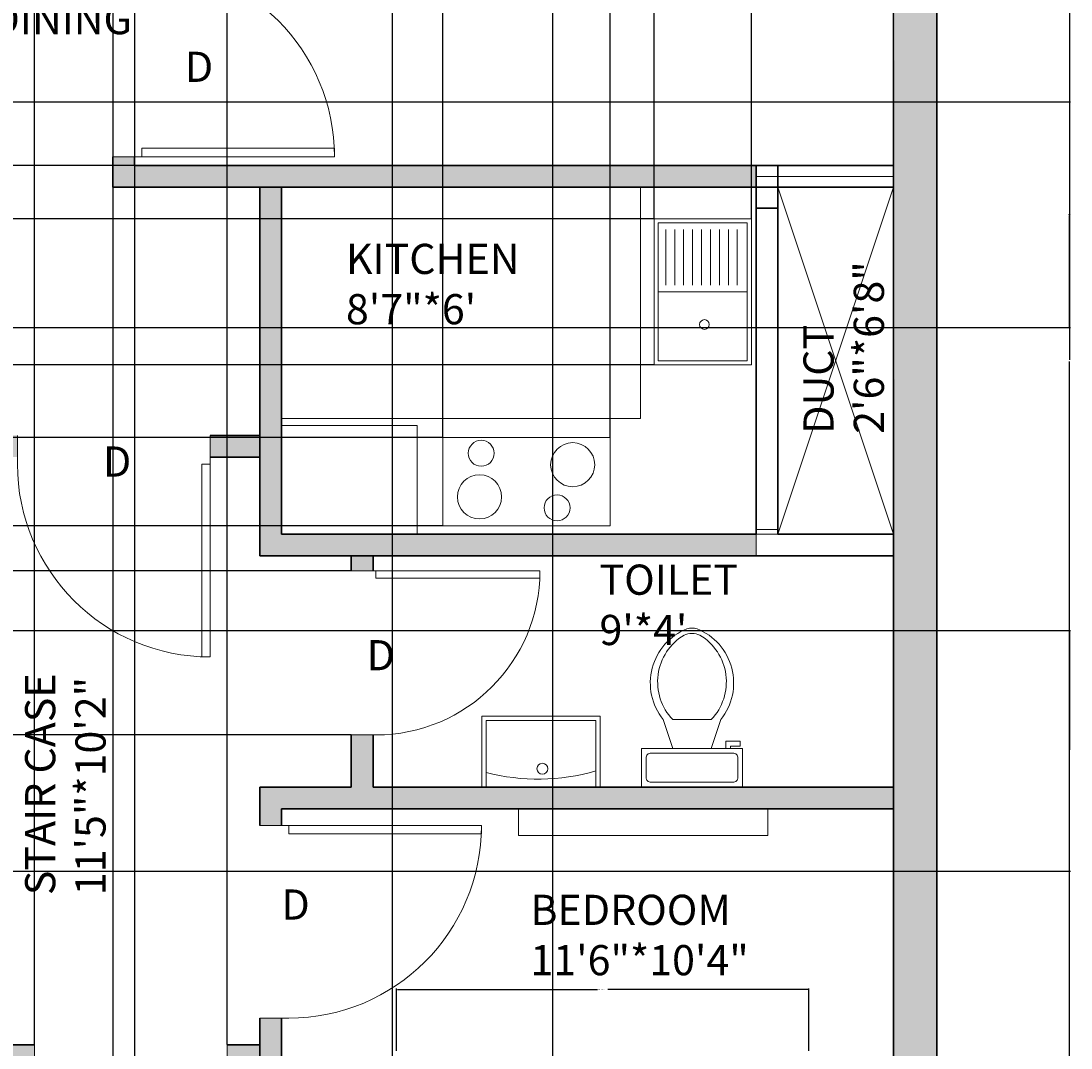
# Model space of a CAD drawing. Units: inches. Extents: x 1841 to 2210, y 2173 to 2736.
# Tile 3 of 4: x 1979 to 2197, y 2316 to 2529. Entities that reach past the tile are written whole.
import ezdxf

# ---------------------------------------------------------------- set-up
doc = ezdxf.new("R2010")
doc.units = ezdxf.units.IN
for name, color, linetype, lineweight in [('A-ANNO-DIMS', 2, 'Continuous', 18), ('A-AREA-IDEN', 10, 'Continuous', 18), ('A-EQPM', 8, 'Continuous', 18), ('A-FLOR-CABN', 8, 'Continuous', 18), ('A-FLOR-FIXT', 9, 'Continuous', 18), ('A-FLOR-FIXT-PATT', 9, 'Continuous', 13), ('A-FLOR-OPEN', 8, 'Continuous', 18), ('A-FURN', 8, 'Continuous', 18), ('A-WALL', 7, 'Continuous', 35), ('A-WALL-PATT', 252, 'Continuous', 13), ('DOOR', 50, 'Continuous', 18), ('TEXT', 10, 'Continuous', 18), ('WIN', 193, 'Continuous', 18)]:
    doc.layers.add(name, color=color, linetype=linetype, lineweight=lineweight)
doc.styles.get("Standard").update_dxf_attribs({"font": 'arial.ttf'})
doc.dimstyles.get("Standard").update_dxf_attribs({"dimtxt": 0.18, "dimasz": 0.18, "dimexe": 0.18, "dimexo": 0.0625, "dimgap": 0.09, "dimtad": 0, "dimtih": 1, "dimtoh": 1, "dimdec": 4, "dimzin": 0, "dimdsep": 46, "dimtxsty": 'Standard', "dimcen": 0.09, "dimadec": 0, "dimazin": 0, "dimtfac": 1, "dimtdec": 4, "dimtofl": 0, "dimtmove": 0, "dimatfit": 3, "dimfxl": 1, "dimtolj": 1, "dimtzin": 0, "dimarcsym": 0})

# ---------------------------------------------------------------- blocks, each defined once
blk = doc.blocks.new('*U2')
for p, q in [((0, 0), (0, -6)), ((40, 0), (40, -6))]:
    blk.add_line(p, q)
blk.add_lwpolyline([(0, 0), (0, 40), (1.75, 40), (1.75, 0)], close=True)
blk.add_arc((0, 0), 40, 0, 90)
blk = doc.blocks.new('*U4')
for p, q in [((9.5, -6), (9.5, -2)), ((-10, -8.5), (-8, -8.5)), ((-10, -9.5), (-10, -8.5)), ((-8, -8.5), (-8, -8)), ((-7, -8), (-7, -9.5)), ((-4, -8), (-6, -14)), ((4, -8), (6, -14)), ((-7, -9.5), (-10, -9.5)), ((4, -14), (-4, -14))]:
    blk.add_line(p, q)
blk.add_lwpolyline([(10.5, -8), (10.5, 0), (-10.5, 0), (-10.5, -8)], close=True)
for points in [[(-9.5, -2), (-9.5, -6)], [(8.5, -1), (-8.5, -1)], [(-8.5, -7), (8.5, -7)]]:
    blk.add_lwpolyline(points)
for centre, radius, start, end in [((-8.62, -1.88), 0.884, 81.8699, 188.1301), ((8.62, -1.88), 0.884, 351.8699, 98.1301), ((-8.62, -6.12), 0.884, 171.8699, 278.1301), ((8.62, -6.12), 0.884, 261.8699, 8.1301), ((3.52, -21.58), 12.17, 141.4691, 247.9714), ((4.2, -21.82), 11.33, 136.3677, 238.9468), ((-3.52, -21.58), 12.17, 292.0284, 38.5307), ((-4.2, -21.82), 11.33, 301.053, 43.6321), ((0, -27.88), 4, 245.7318, 294.2682), ((0, -29), 4, 254.8605, 285.1395)]:
    blk.add_arc(centre, radius, start, end)
blk = doc.blocks.new('BASIN-WALL')
blk.add_lwpolyline([(24.58, 14.71), (24.58, 0), (0, 0), (0, 14.71)])
blk.add_lwpolyline([(0.91, 14.71), (23.68, 14.71), (23.68, 0.91), (0.91, 0.91)], close=True)
blk.add_circle((11.97, 10.91), 1.13)
blk.add_arc((12.85, -29.32), 42.4, 75.2054, 106.3847)
blk = doc.blocks.new('*D16')
at = {"layer": 'A-ANNO-DIMS', "color": 0, "lineweight": -2, "transparency": 16777216}
for p, q in [((2056.93, 2315.11), (2056.93, 2328.07)), ((2057.11, 2327.89), (2098.62, 2327.89)), ((2142.32, 2327.89), (2100.81, 2327.89)), ((2142.5, 2315.11), (2142.5, 2328.07))]:
    blk.add_line(p, q, dxfattribs=at)
at = {"layer": 'A-ANNO-DIMS', "color": 0, "transparency": 16777216}
for points in [[(2057.11, 2327.92), (2057.11, 2327.86), (2056.93, 2327.89)], [(2142.32, 2327.92), (2142.32, 2327.86), (2142.5, 2327.89)]]:
    blk.add_solid(points, dxfattribs=at)
at = {"layer": 'Defpoints', "color": 0, "transparency": 16777216}
for p in [(2056.93, 2327.89), (2056.93, 2315.05), (2142.5, 2315.05)]:
    blk.add_point(p, dxfattribs=at)
at = {"layer": 'A-ANNO-DIMS', "color": 0, "transparency": 16777216, "insert": (2099.72, 2327.89), "char_height": 0.18, "attachment_point": 5}
blk.add_mtext('\\A1;BED SET 86 TYP.', dxfattribs=at)
blk = doc.blocks.new('*D23')
at = {"layer": 'A-ANNO-DIMS', "color": 0, "lineweight": -2, "transparency": 16777216}
for p, q in [((2169.11, 2708.41), (2196.78, 2708.41)), ((2196.6, 2708.23), (2196.6, 2458.59)), ((2196.6, 2208.59), (2196.6, 2458.22)), ((2028.61, 2208.41), (2196.78, 2208.41))]:
    blk.add_line(p, q, dxfattribs=at)
at = {"layer": 'A-ANNO-DIMS', "color": 0, "transparency": 16777216}
for points in [[(2196.57, 2708.23), (2196.63, 2708.23), (2196.6, 2708.41)], [(2196.57, 2208.59), (2196.63, 2208.59), (2196.6, 2208.41)]]:
    blk.add_solid(points, dxfattribs=at)
at = {"layer": 'Defpoints', "color": 0, "transparency": 16777216}
for p in [(2169.05, 2708.41), (2196.6, 2708.41), (2028.55, 2208.41)]:
    blk.add_point(p, dxfattribs=at)
at = {"layer": 'A-ANNO-DIMS', "color": 0, "transparency": 16777216, "insert": (2196.6, 2458.41), "char_height": 0.18, "attachment_point": 5}
blk.add_mtext('\\A1;500', dxfattribs=at)
blk = doc.blocks.new('*D35')
at = {"layer": 'A-ANNO-DIMS', "color": 0, "lineweight": -2, "transparency": 16777216}
for p, q in [((2159.99, 2546.82), (1841.32, 2546.82)), ((1841.5, 2546.64), (1841.5, 2523.04)), ((1841.5, 2499.09), (1841.5, 2522.68)), ((2159.99, 2498.91), (1841.32, 2498.91))]:
    blk.add_line(p, q, dxfattribs=at)
at = {"layer": 'A-ANNO-DIMS', "color": 0, "transparency": 16777216}
for points in [[(1841.47, 2546.64), (1841.53, 2546.64), (1841.5, 2546.82)], [(1841.47, 2499.09), (1841.53, 2499.09), (1841.5, 2498.91)]]:
    blk.add_solid(points, dxfattribs=at)
at = {"layer": 'Defpoints', "color": 0, "transparency": 16777216}
for p in [(1841.5, 2546.82), (2160.05, 2546.82), (2160.05, 2498.91)]:
    blk.add_point(p, dxfattribs=at)
at = {"layer": 'A-ANNO-DIMS', "color": 0, "transparency": 16777216, "insert": (1841.5, 2522.86), "char_height": 0.18, "attachment_point": 5}
blk.add_mtext('\\A1;47.91', dxfattribs=at)
blk = doc.blocks.new('*D36')
at = {"layer": 'A-ANNO-DIMS', "color": 0, "lineweight": -2, "transparency": 16777216}
for p, q in [((1981.8, 2316.47), (1981.8, 2736.14)), ((1981.98, 2735.96), (2001.58, 2735.96)), ((2021.62, 2735.96), (2002.02, 2735.96)), ((2021.8, 2316.47), (2021.8, 2736.14))]:
    blk.add_line(p, q, dxfattribs=at)
at = {"layer": 'A-ANNO-DIMS', "color": 0, "transparency": 16777216}
for points in [[(1981.98, 2735.99), (1981.98, 2735.93), (1981.8, 2735.96)], [(2021.62, 2735.99), (2021.62, 2735.93), (2021.8, 2735.96)]]:
    blk.add_solid(points, dxfattribs=at)
at = {"layer": 'Defpoints', "color": 0, "transparency": 16777216}
for p in [(2021.8, 2735.96), (1981.8, 2316.41), (2021.8, 2316.41)]:
    blk.add_point(p, dxfattribs=at)
at = {"layer": 'A-ANNO-DIMS', "color": 0, "transparency": 16777216, "insert": (2001.8, 2735.96), "char_height": 0.18, "attachment_point": 5}
blk.add_mtext('\\A1;40', dxfattribs=at)
blk = doc.blocks.new('*D39')
at = {"layer": 'A-ANNO-DIMS', "color": 0, "lineweight": -2, "transparency": 16777216}
for p, q in [((1914.11, 2402.41), (2196.78, 2402.41)), ((2196.6, 2402.23), (2196.6, 2377.59)), ((2196.6, 2352.59), (2196.6, 2377.22)), ((1914.11, 2352.41), (2196.78, 2352.41))]:
    blk.add_line(p, q, dxfattribs=at)
at = {"layer": 'A-ANNO-DIMS', "color": 0, "transparency": 16777216}
for points in [[(2196.57, 2402.23), (2196.63, 2402.23), (2196.6, 2402.41)], [(2196.57, 2352.59), (2196.63, 2352.59), (2196.6, 2352.41)]]:
    blk.add_solid(points, dxfattribs=at)
at = {"layer": 'Defpoints', "color": 0, "transparency": 16777216}
for p in [(1914.05, 2402.41), (2196.6, 2402.41), (1914.05, 2352.41)]:
    blk.add_point(p, dxfattribs=at)
at = {"layer": 'A-ANNO-DIMS', "color": 0, "transparency": 16777216, "insert": (2196.6, 2377.41), "char_height": 0.18, "attachment_point": 5}
blk.add_mtext('\\A1;50', dxfattribs=at)
blk = doc.blocks.new('*D41')
at = {"layer": 'A-ANNO-DIMS', "color": 0, "lineweight": -2, "transparency": 16777216}
for p, q in [((1938.73, 2512.15), (2196.78, 2512.15)), ((2196.6, 2511.97), (2196.6, 2488.89)), ((2196.6, 2465.46), (2196.6, 2488.53)), ((1938.73, 2465.28), (2196.78, 2465.28))]:
    blk.add_line(p, q, dxfattribs=at)
at = {"layer": 'A-ANNO-DIMS', "color": 0, "transparency": 16777216}
for points in [[(2196.57, 2511.97), (2196.63, 2511.97), (2196.6, 2512.15)], [(2196.57, 2465.46), (2196.63, 2465.46), (2196.6, 2465.28)]]:
    blk.add_solid(points, dxfattribs=at)
at = {"layer": 'Defpoints', "color": 0, "transparency": 16777216}
for p in [(1938.67, 2512.15), (2196.6, 2512.15), (1938.67, 2465.28)]:
    blk.add_point(p, dxfattribs=at)
at = {"layer": 'A-ANNO-DIMS', "color": 0, "transparency": 16777216, "insert": (2196.6, 2488.71), "char_height": 0.18, "attachment_point": 5}
blk.add_mtext('\\A1;46.87', dxfattribs=at)
blk = doc.blocks.new('*D43')
at = {"layer": 'A-ANNO-DIMS', "color": 0, "lineweight": -2, "transparency": 16777216}
for p, q in [((2056.06, 2637.84), (2056.06, 2180.68)), ((2089.3, 2637.84), (2089.3, 2180.68)), ((2056.24, 2180.86), (2072.22, 2180.86)), ((2089.12, 2180.86), (2073.14, 2180.86))]:
    blk.add_line(p, q, dxfattribs=at)
at = {"layer": 'A-ANNO-DIMS', "color": 0, "transparency": 16777216}
for points in [[(2056.24, 2180.89), (2056.24, 2180.83), (2056.06, 2180.86)], [(2089.12, 2180.89), (2089.12, 2180.83), (2089.3, 2180.86)]]:
    blk.add_solid(points, dxfattribs=at)
at = {"layer": 'Defpoints', "color": 0, "transparency": 16777216}
for p in [(2056.06, 2637.91), (2089.3, 2637.91), (2089.3, 2180.86)]:
    blk.add_point(p, dxfattribs=at)
at = {"layer": 'A-ANNO-DIMS', "color": 0, "transparency": 16777216, "insert": (2072.68, 2180.86), "char_height": 0.18, "attachment_point": 5}
blk.add_mtext('\\A1;33.234', dxfattribs=at)
blk = doc.blocks.new('*D44')
at = {"layer": 'A-ANNO-DIMS', "color": 0, "lineweight": -2, "transparency": 16777216}
for p, q in [((2047.49, 2414.75), (1841.32, 2414.75)), ((1841.5, 2414.57), (1841.5, 2397.92)), ((1841.5, 2380.9), (1841.5, 2397.56)), ((2047.49, 2380.72), (1841.32, 2380.72))]:
    blk.add_line(p, q, dxfattribs=at)
at = {"layer": 'A-ANNO-DIMS', "color": 0, "transparency": 16777216}
for points in [[(1841.47, 2414.57), (1841.53, 2414.57), (1841.5, 2414.75)], [(1841.47, 2380.9), (1841.53, 2380.9), (1841.5, 2380.72)]]:
    blk.add_solid(points, dxfattribs=at)
at = {"layer": 'Defpoints', "color": 0, "transparency": 16777216}
for p in [(1841.5, 2414.75), (2047.55, 2414.75), (2047.55, 2380.72)]:
    blk.add_point(p, dxfattribs=at)
at = {"layer": 'A-ANNO-DIMS', "color": 0, "transparency": 16777216, "insert": (1841.5, 2397.74), "char_height": 0.18, "attachment_point": 5}
blk.add_mtext('\\A1;34.03', dxfattribs=at)
blk = doc.blocks.new('*D45')
at = {"layer": 'A-ANNO-DIMS', "color": 0, "lineweight": -2, "transparency": 16777216}
for p, q in [((1998.05, 2540.69), (1998.05, 2180.68)), ((2002.55, 2540.69), (2002.55, 2180.68)), ((1998.23, 2180.86), (2000.04, 2180.86)), ((2002.37, 2180.86), (2000.56, 2180.86))]:
    blk.add_line(p, q, dxfattribs=at)
at = {"layer": 'A-ANNO-DIMS', "color": 0, "transparency": 16777216}
for points in [[(1998.23, 2180.89), (1998.23, 2180.83), (1998.05, 2180.86)], [(2002.37, 2180.89), (2002.37, 2180.83), (2002.55, 2180.86)]]:
    blk.add_solid(points, dxfattribs=at)
at = {"layer": 'Defpoints', "color": 0, "transparency": 16777216}
for p in [(1998.05, 2540.75), (2002.55, 2540.75), (2002.55, 2180.86)]:
    blk.add_point(p, dxfattribs=at)
at = {"layer": 'A-ANNO-DIMS', "color": 0, "transparency": 16777216, "insert": (2000.3, 2180.86), "char_height": 0.18, "attachment_point": 5}
blk.add_mtext('\\A1;4.5', dxfattribs=at)
blk = doc.blocks.new('*D47')
at = {"layer": 'A-ANNO-DIMS', "color": 0, "lineweight": -2, "transparency": 16777216}
for p, q in [((2066.54, 2442.55), (2066.54, 2736.14)), ((2066.72, 2735.96), (2083.52, 2735.96)), ((2101.11, 2735.96), (2084.31, 2735.96)), ((2101.29, 2442.55), (2101.29, 2736.14))]:
    blk.add_line(p, q, dxfattribs=at)
at = {"layer": 'A-ANNO-DIMS', "color": 0, "transparency": 16777216}
for points in [[(2066.72, 2735.99), (2066.72, 2735.93), (2066.54, 2735.96)], [(2101.11, 2735.99), (2101.11, 2735.93), (2101.29, 2735.96)]]:
    blk.add_solid(points, dxfattribs=at)
at = {"layer": 'Defpoints', "color": 0, "transparency": 16777216}
for p in [(2101.29, 2735.96), (2066.54, 2442.49), (2101.29, 2442.49)]:
    blk.add_point(p, dxfattribs=at)
at = {"layer": 'A-ANNO-DIMS', "color": 0, "transparency": 16777216, "insert": (2083.91, 2735.96), "char_height": 0.18, "attachment_point": 5}
blk.add_mtext('\\A1;34.75', dxfattribs=at)
blk = doc.blocks.new('*D48')
at = {"layer": 'A-ANNO-DIMS', "color": 0, "lineweight": -2, "transparency": 16777216}
for p, q in [((2066.48, 2442.49), (1841.32, 2442.49)), ((1841.5, 2442.31), (1841.5, 2433.48)), ((1841.5, 2424.29), (1841.5, 2433.12)), ((2066.48, 2424.11), (1841.32, 2424.11))]:
    blk.add_line(p, q, dxfattribs=at)
at = {"layer": 'A-ANNO-DIMS', "color": 0, "transparency": 16777216}
for points in [[(1841.47, 2442.31), (1841.53, 2442.31), (1841.5, 2442.49)], [(1841.47, 2424.29), (1841.53, 2424.29), (1841.5, 2424.11)]]:
    blk.add_solid(points, dxfattribs=at)
at = {"layer": 'Defpoints', "color": 0, "transparency": 16777216}
for p in [(1841.5, 2442.49), (2066.54, 2442.49), (2066.54, 2424.11)]:
    blk.add_point(p, dxfattribs=at)
at = {"layer": 'A-ANNO-DIMS', "color": 0, "transparency": 16777216, "insert": (1841.5, 2433.3), "char_height": 0.18, "attachment_point": 5}
blk.add_mtext('\\A1;18.377', dxfattribs=at)
blk = doc.blocks.new('*D49')
at = {"layer": 'A-ANNO-DIMS', "color": 0, "lineweight": -2, "transparency": 16777216}
for p, q in [((2110.38, 2487.94), (2110.38, 2736.14)), ((2110.56, 2735.96), (2120.1, 2735.96)), ((2130.41, 2735.96), (2120.86, 2735.96)), ((2130.59, 2487.94), (2130.59, 2736.14))]:
    blk.add_line(p, q, dxfattribs=at)
at = {"layer": 'A-ANNO-DIMS', "color": 0, "transparency": 16777216}
for points in [[(2110.56, 2735.99), (2110.56, 2735.93), (2110.38, 2735.96)], [(2130.41, 2735.99), (2130.41, 2735.93), (2130.59, 2735.96)]]:
    blk.add_solid(points, dxfattribs=at)
at = {"layer": 'Defpoints', "color": 0, "transparency": 16777216}
for p in [(2130.59, 2735.96), (2110.38, 2487.88), (2130.59, 2487.88)]:
    blk.add_point(p, dxfattribs=at)
at = {"layer": 'A-ANNO-DIMS', "color": 0, "transparency": 16777216, "insert": (2120.48, 2735.96), "char_height": 0.18, "attachment_point": 5}
blk.add_mtext('\\A1;20.21', dxfattribs=at)
blk = doc.blocks.new('*D50')
at = {"layer": 'A-ANNO-DIMS', "color": 0, "lineweight": -2, "transparency": 16777216}
for p, q in [((2110.31, 2487.88), (1841.32, 2487.88)), ((1841.5, 2487.7), (1841.5, 2472.88)), ((1841.5, 2457.7), (1841.5, 2472.52)), ((2110.31, 2457.52), (1841.32, 2457.52))]:
    blk.add_line(p, q, dxfattribs=at)
at = {"layer": 'A-ANNO-DIMS', "color": 0, "transparency": 16777216}
for points in [[(1841.47, 2487.7), (1841.53, 2487.7), (1841.5, 2487.88)], [(1841.47, 2457.7), (1841.53, 2457.7), (1841.5, 2457.52)]]:
    blk.add_solid(points, dxfattribs=at)
at = {"layer": 'Defpoints', "color": 0, "transparency": 16777216}
for p in [(1841.5, 2487.88), (2110.38, 2487.88), (2110.38, 2457.52)]:
    blk.add_point(p, dxfattribs=at)
at = {"layer": 'A-ANNO-DIMS', "color": 0, "transparency": 16777216, "insert": (1841.5, 2472.7), "char_height": 0.18, "attachment_point": 5}
blk.add_mtext('\\A1;30.36', dxfattribs=at)

msp = doc.modelspace()

# ---------------------------------------------------------------- hatches: boundary and pattern name
at = {"layer": 'A-FLOR-FIXT-PATT'}
h = msp.add_hatch(dxfattribs=at)
h.set_pattern_fill('ANSI31', color=256, scale=0.5842426, angle=45, style=0)
h.paths.add_polyline_path([(2112.5297, 2474.0845), (2128.2451, 2474.0845), (2128.2451, 2485.6514), (2112.5297, 2485.6514)])
at = {"layer": 'A-WALL-PATT'}
h = msp.add_hatch(color=256, dxfattribs=at)
h.dxf.hatch_style = 1
h.paths.add_polyline_path([(2169.0509, 2546.8192), (2160.3559, 2546.8192), (2160.3559, 2545.451), (2160.3559, 2529.1476), (2160.0509, 2237.4052), (2128.1686, 2237.4052), (2128.1686, 2228.4052), (2169.0509, 2228.4052)])
h.paths.add_polyline_path([(2067.6527, 2237.4052), (2028.5509, 2237.4052), (2028.5509, 2228.4052), (2067.6527, 2228.4052)])
h.paths.add_polyline_path([(2033.0509, 2321.9228), (2028.5509, 2321.9228), (2028.5509, 2237.4052), (2033.0509, 2237.4052)])
h.paths.add_polyline_path([(2160.0509, 2369.9052), (2052.0509, 2369.9052), (2052.0509, 2380.7227), (2047.5509, 2380.7227), (2047.5509, 2369.9052), (2028.5509, 2369.9052), (2028.5509, 2364.1588), (2028.5509, 2361.9228), (2033.0509, 2361.9228), (2033.0509, 2365.4052), (2050.3181, 2365.4052), (2160.0509, 2365.4052)])
h.paths.add_polyline_path([(1878.0509, 2346.5722), (1869.0509, 2346.5722), (1869.0509, 2228.4052), (1878.0509, 2228.4052), (1878.0509, 2237.4052)])
h.paths.add_polyline_path([(1981.8009, 2316.4052), (1878.0509, 2316.4052), (1878.0509, 2311.9052), (1981.8009, 2311.9052)])
h.paths.add_polyline_path([(1978.2584, 2442.9052), (1878.0509, 2442.9052), (1878.0509, 2438.4052), (1914.0509, 2438.4052), (1978.2584, 2438.4052)])
h.paths.add_polyline_path([(1878.0509, 2468.4052), (1869.0509, 2468.4052), (1869.0509, 2407.0881), (1878.0509, 2407.0881), (1878.0509, 2438.4052)])
h.paths.add_polyline_path([(2028.5509, 2442.9052), (2018.2584, 2442.9052), (2018.2584, 2438.4052), (2028.5509, 2438.4052)])
h.paths.add_polyline_path([(2131.5968, 2498.9052), (2002.5509, 2498.9052), (2002.5509, 2500.7487), (1998.0509, 2500.7487), (1998.0509, 2494.4052), (2131.5968, 2494.4052)])
h.paths.add_polyline_path([(2033.0509, 2489.9052), (2033.0509, 2494.4052), (2028.5509, 2494.4052), (2028.5509, 2489.9052), (2028.5509, 2417.9052), (2131.5509, 2417.9052), (2131.5509, 2422.4052), (2033.0509, 2422.4052), (2033.0294, 2446.4052)])
h.paths.add_polyline_path([(1953.1667, 2555.4052), (1878.0509, 2555.4052), (1878.0509, 2550.9052), (1953.1667, 2550.9052)], flags=17)
h.paths.add_polyline_path([(1878.0509, 2699.4052), (2160.0509, 2699.4052), (2160.0509, 2607.3351), (2169.0509, 2607.3351), (2169.0509, 2708.4052), (1869.0509, 2708.4052), (1869.0509, 2528.9211), (1878.0509, 2528.9211), (1878.0509, 2550.9052), (1878.0509, 2555.4052)])
h.paths.add_polyline_path([(1998.0509, 2555.4052), (1993.1667, 2555.4052), (1993.1667, 2550.9052), (1998.0509, 2550.9052)], flags=17)
h.paths.add_polyline_path([(2002.5509, 2550.9052), (1998.0509, 2550.9052), (1998.0509, 2540.7487), (2002.5509, 2540.7487)], flags=17)
h.paths.add_polyline_path([(2002.5509, 2576.8157), (2002.5509, 2607.2805), (2002.5509, 2699.4052), (1998.0509, 2699.4052), (1998.0509, 2555.4052), (1998.0509, 2550.9052), (2002.5509, 2550.9052)], flags=17)
h.paths.add_polyline_path([(2160.0509, 2642.4052), (2089.2965, 2642.4052), (2089.2965, 2637.9052), (2160.0509, 2637.9052)], flags=17)
h.paths.add_polyline_path([(2056.0629, 2642.4052), (2054.0509, 2642.4052), (2054.0509, 2699.4052), (2049.5509, 2699.4052), (2049.5509, 2642.4052), (2002.5509, 2642.4052), (2002.5509, 2637.9052), (2054.0509, 2637.9052), (2056.0629, 2637.9052)], flags=17)
h.paths.add_polyline_path([(1924.594, 2243.1802), (1965.0263, 2243.1802), (1965.0263, 2266.5581), (1924.594, 2266.5581)], flags=9)
h.paths.add_polyline_path([(2082.2056, 2327.2752), (2130.8731, 2327.2752), (2130.8731, 2350.6531), (2082.2056, 2350.6531)], flags=9)
h.paths.add_polyline_path([(2000.1077, 2344.9343), (2000.1077, 2400.666), (1976.7298, 2400.666), (1976.7298, 2344.9343)], flags=9)
h.paths.add_polyline_path([(2161.6353, 2440.9897), (2161.6353, 2476.9732), (2138.2574, 2476.9732), (2138.2574, 2440.9897)], flags=24)
h.paths.add_polyline_path([(2044.2273, 2462.409), (2085.775, 2462.409), (2085.775, 2485.7869), (2044.2273, 2485.7869)], flags=25)
h.paths.add_polyline_path([(1940.3738, 2512.1813), (2005.58, 2512.1813), (2005.58, 2535.5592), (1940.3738, 2535.5592)], flags=9)
h.paths.add_polyline_path([(2088.5551, 2604.7497), (2142.0901, 2604.7497), (2142.0901, 2628.1276), (2088.5551, 2628.1276)], flags=25)
h.paths.add_polyline_path([(2110.3045, 2670.6273), (2145.8692, 2670.6273), (2145.8692, 2694.0052), (2110.3045, 2694.0052)], flags=25)
h.paths.add_polyline_path([(2002.7596, 2670.6273), (2043.2176, 2670.6273), (2043.2176, 2694.0052), (2002.7596, 2694.0052)], flags=24)
h.paths.add_polyline_path([(1907.1501, 2670.6273), (1955.8175, 2670.6273), (1955.8175, 2694.0052), (1907.1501, 2694.0052)], flags=25)
h = msp.add_hatch(color=256, dxfattribs=at)
h.dxf.hatch_style = 1
h.paths.add_polyline_path([(2028.5509, 2316.4052), (2021.8009, 2316.4052), (2021.8009, 2311.9052), (2028.5509, 2311.9052)])
h.paths.add_polyline_path([(2052.0509, 2417.9052), (2047.5509, 2417.9052), (2047.5509, 2414.752), (2052.0509, 2414.752)])

# ---------------------------------------------------------------- linework, layer by layer
at = {"layer": 'A-EQPM'}
msp.add_lwpolyline([(2066.5401, 2424.1127), (2101.2887, 2424.1127), (2101.2887, 2442.4893), (2066.5401, 2442.4893)], close=True, dxfattribs=at)
for centre, radius in [((2074.5068, 2439.1866), 2.6934), ((2093.4915, 2436.8154), 4.5766), ((2074.1678, 2430.1253), 4.5766), ((2090.2462, 2427.8552), 2.6934)]:
    msp.add_circle(centre, radius, dxfattribs=at)
at = {"layer": 'A-FLOR-CABN'}
for p, q in [((2131.5968, 2494.4052), (2107.5968, 2494.4052)), ((2107.5968, 2494.4052), (2107.5968, 2446.4052)), ((2033.0509, 2422.4052), (2033.0294, 2446.4052)), ((2033.0294, 2446.4052), (2107.5968, 2446.4052))]:
    msp.add_line(p, q, dxfattribs=at)
msp.add_lwpolyline([(2033.0509, 2422.4052), (2061.1901, 2422.4052), (2061.1901, 2444.9637), (2033.0509, 2444.9637)], close=True, dxfattribs=at)
at = {"layer": 'A-FLOR-FIXT'}
msp.add_line((2129.716, 2472.7004), (2111.2459, 2472.7004), dxfattribs=at)
for points in [[(2110.3763, 2457.5216), (2130.5857, 2457.5216), (2130.5857, 2487.8791), (2110.3763, 2487.8791)], [(2111.2459, 2458.3913), (2129.716, 2458.3913), (2129.716, 2487.0094), (2111.2459, 2487.0094)]]:
    msp.add_lwpolyline(points, close=True, dxfattribs=at)
msp.add_circle((2120.8387, 2465.9134), 1.009, dxfattribs=at)
at = {"layer": 'A-FLOR-OPEN'}
for p, q in [((2136.0509, 2422.4052), (2160.0509, 2494.4052)), ((2136.0509, 2494.4052), (2160.0509, 2422.4052))]:
    msp.add_line(p, q, dxfattribs=at)
at = {"layer": 'A-FURN'}
msp.add_lwpolyline([(2082.263, 2365.4052), (2133.9973, 2365.4052), (2133.9973, 2359.8207), (2082.263, 2359.8207)], close=True, dxfattribs=at)
at = {"layer": 'A-WALL'}
for p, q in [((2160.0509, 2637.9052), (2160.0509, 2498.9052)), ((1998.0509, 2494.4052), (1998.0509, 2500.7487)), ((2002.5509, 2498.9052), (2002.5509, 2500.7487)), ((2160.0509, 2498.9052), (2002.5509, 2498.9052)), ((2160.0509, 2494.4052), (1998.0509, 2494.4052)), ((2028.5509, 2489.9052), (2028.5509, 2494.4052)), ((2033.0509, 2489.9052), (2033.0509, 2494.4052)), ((2131.5509, 2422.4052), (2131.5509, 2494.4052)), ((2136.0509, 2422.4052), (2136.0509, 2494.4052)), ((2160.0509, 2494.4052), (2160.0509, 2422.4052)), ((2028.5509, 2417.9052), (2028.5509, 2489.9052)), ((2033.0509, 2422.4052), (2033.0509, 2489.9052)), ((2018.2584, 2442.9052), (2028.5509, 2442.9052)), ((2018.2584, 2438.4052), (2028.5509, 2438.4052)), ((2131.5509, 2422.4052), (2033.0509, 2422.4052)), ((2160.0509, 2422.4052), (2136.0509, 2422.4052)), ((2131.5509, 2417.9052), (2028.5509, 2417.9052)), ((2047.5509, 2414.752), (2047.5509, 2417.9052)), ((2052.0509, 2414.752), (2052.0509, 2417.9052)), ((2160.0509, 2417.9052), (2131.5509, 2417.9052)), ((2160.0509, 2417.9052), (2160.0509, 2369.9052)), ((2047.5509, 2369.9052), (2047.5509, 2380.7227)), ((2052.0509, 2369.9052), (2052.0509, 2380.7227)), ((2047.5509, 2369.9052), (2028.5509, 2369.9052)), ((2028.5509, 2369.9052), (2028.5509, 2364.1588)), ((2160.0509, 2369.9052), (2052.0509, 2369.9052)), ((2028.5509, 2365.4052), (2028.5509, 2361.9228)), ((2033.0509, 2365.4052), (2050.3181, 2365.4052)), ((2033.0509, 2365.4052), (2033.0509, 2361.9228)), ((2160.0509, 2365.4052), (2047.5509, 2365.4052)), ((2028.5509, 2321.9228), (2028.5509, 2237.4052)), ((2033.0509, 2321.9228), (2033.0509, 2237.4052)), ((1878.0509, 2316.4052), (1981.8009, 2316.4052)), ((2021.8009, 2316.4052), (2028.5509, 2316.4052))]:
    msp.add_line(p, q, dxfattribs=at)
for points in [[(1869.0509, 2228.4052), (2169.0509, 2228.4052), (2169.0509, 2708.4052), (1869.0509, 2708.4052)], [(2136.0509, 2490.049), (2131.5968, 2490.049), (2131.5968, 2498.9052), (2136.0509, 2498.9052)]]:
    msp.add_lwpolyline(points, close=True, dxfattribs=at)
msp.add_lwpolyline([(2028.5509, 2237.4052), (2160.0509, 2237.4052), (2160.0509, 2699.4052), (1878.0509, 2699.4052), (1878.0509, 2237.4052)], dxfattribs=at)
at = {"layer": 'WIN'}
msp.add_line((2131.5968, 2496.6552), (2160.0509, 2496.6552), dxfattribs=at)
for points in [[(2131.5509, 2494.4771), (2160.0509, 2494.4771), (2160.0509, 2498.9052), (2131.5509, 2498.9052)], [(2131.5968, 2494.4052), (2160.0509, 2494.4052), (2160.0509, 2498.9052), (2131.5968, 2498.9052)], [(2131.5509, 2423.3797), (2136.0509, 2423.3797), (2136.0509, 2494.4771), (2131.5509, 2494.4771)], [(2131.5509, 2417.9052), (2160.0509, 2417.9052), (2160.0509, 2422.4052), (2131.5509, 2422.4052)]]:
    msp.add_lwpolyline(points, close=True, dxfattribs=at)

# ---------------------------------------------------------------- block references
at = {"layer": 'A-FLOR-FIXT', "rotation": 180}
for name, p in [('*U4', (2118.2505, 2369.9052)), ('BASIN-WALL', (2099.1825, 2384.6164))]:
    msp.add_blockref(name, p, dxfattribs=at)
at = {"layer": 'DOOR', "xscale": -1, "rotation": 270}
msp.add_blockref('*U2', (2004.0509, 2500.7487), dxfattribs=at)
at = {"layer": 'DOOR'}
for p, rotation in [((2018.2584, 2436.9052), 180), ((2034.5509, 2361.9228), 270), ((2021.8009, 2310.4052), 180)]:
    msp.add_blockref('*U2', p, dxfattribs=dict(at, rotation=rotation))
at = {"layer": 'DOOR', "xscale": 0.8507339676805603, "yscale": 0.8507339676805603, "zscale": 0.8507339676805603, "rotation": 270}
msp.add_blockref('*U2', (2052.6553, 2414.752), dxfattribs=at)

# ---------------------------------------------------------------- texts
at = {"layer": 'A-AREA-IDEN', "char_height": 6.26506, "attachment_point": 1}
for s, insert in [("LIVING/DINING\\P10'*9'", (1942.893, 2532.4416)), ('KITCHEN\\P8\'7"*6\'', (2046.4346, 2482.6693)), ("TOILET\\P9'*4'", (2099.0553, 2416.0791)), ('BEDROOM\\P11\'6"*10\'4"', (2084.7249, 2347.5398))]:
    msp.add_mtext_dynamic_manual_height_columns(s, width=112.651532, gutter_width=31.3253, heights=[0], dxfattribs=dict(at, insert=insert))
at = {"layer": 'A-AREA-IDEN', "char_height": 6.26506, "attachment_point": 1, "rotation": 90}
for s, insert in [('DUCT\\P2\'6"*6\'8"', (2141.375, 2443.2312)), ('STAIR CASE\\P11\'5"*10\'2"', (1979.8474, 2347.4536))]:
    msp.add_mtext_dynamic_manual_height_columns(s, width=112.651532, gutter_width=31.3253, heights=[0], dxfattribs=dict(at, insert=insert))
at = {"layer": 'TEXT', "char_height": 6.2651, "attachment_point": 1}
for insert in [(2013.0041, 2522.5407), (1996.0033, 2440.5952), (2050.726, 2400.4002), (2033.0464, 2348.6378)]:
    msp.add_mtext_dynamic_manual_height_columns('D', width=112.651532, gutter_width=31.3253, heights=[0], dxfattribs=dict(at, insert=insert))

# ---------------------------------------------------------------- dimensions: what is measured, and where the dimension line sits
at = {"layer": 'A-ANNO-DIMS'}
for base, p1, p2, override, picture, middle in [((2021.8009, 2735.9552), (1981.8009, 2316.4052), (2021.8009, 2316.4052), {"dimdec": 0, "dimlfac": 1, "dimrnd": 0, "dimzin": 0, "dimdsep": 46, "dimlunit": 2}, '*D36', (2001.8009, 2735.9552)), ((2101.2887, 2735.9552), (2066.5401, 2442.4893), (2101.2887, 2442.4893), {"dimdec": 2, "dimlfac": 1, "dimrnd": 0, "dimzin": 0, "dimdsep": 46, "dimlunit": 2}, '*D47', (2083.9144, 2735.9552)), ((2130.5857, 2735.9552), (2110.3763, 2487.8791), (2130.5857, 2487.8791), {"dimdec": 2, "dimlfac": 1, "dimrnd": 0, "dimzin": 0, "dimdsep": 46, "dimlunit": 2}, '*D49', (2120.481, 2735.9552)), ((2089.2965, 2180.8552), (2056.0629, 2637.9052), (2089.2965, 2637.9052), {"dimdec": 3, "dimlfac": 1, "dimrnd": 0, "dimzin": 0, "dimdsep": 46, "dimlunit": 2}, '*D43', (2072.6797, 2180.8552)), ((2002.5509, 2180.8552), (1998.0509, 2540.7487), (2002.5509, 2540.7487), {"dimdec": 1, "dimlfac": 1, "dimrnd": 0, "dimzin": 0, "dimdsep": 46, "dimlunit": 2}, '*D45', (2000.3009, 2180.8552))]:
    dim = msp.add_linear_dim(base=base, p1=p1, p2=p2, dimstyle='Standard', override=override, dxfattribs=at)
    dim.commit()
    dim.dimension.update_dxf_attribs({"geometry": picture, "text_midpoint": middle})
for base, p1, p2, override, picture, middle in [((2196.6009, 2708.4052), (2028.5509, 2208.4052), (2169.0509, 2708.4052), {"dimdec": 0, "dimlfac": 1, "dimrnd": 0, "dimzin": 0, "dimdsep": 46, "dimlunit": 2}, '*D23', (2196.6009, 2458.4052)), ((1841.5009, 2546.8192), (2160.0509, 2498.9052), (2160.0509, 2546.8192), {"dimdec": 2, "dimlfac": 1, "dimrnd": 0, "dimzin": 0, "dimdsep": 46, "dimlunit": 2}, '*D35', (1841.5009, 2522.8622)), ((2196.6009, 2512.1455), (1938.6659, 2465.2791), (1938.6659, 2512.1455), {"dimdec": 2, "dimlfac": 1, "dimrnd": 0, "dimzin": 0, "dimdsep": 46, "dimlunit": 2}, '*D41', (2196.6009, 2488.7123)), ((1841.5009, 2487.8791), (2110.3763, 2457.5216), (2110.3763, 2487.8791), {"dimdec": 2, "dimlfac": 1, "dimrnd": 0, "dimzin": 0, "dimdsep": 46, "dimlunit": 2}, '*D50', (1841.5009, 2472.7004)), ((1841.5009, 2442.4893), (2066.5401, 2424.1127), (2066.5401, 2442.4893), {"dimdec": 3, "dimlfac": 1, "dimrnd": 0, "dimzin": 0, "dimdsep": 46, "dimlunit": 2}, '*D48', (1841.5009, 2433.301)), ((1841.5009, 2414.752), (2047.5509, 2380.7227), (2047.5509, 2414.752), {"dimdec": 2, "dimlfac": 1, "dimrnd": 0, "dimzin": 0, "dimdsep": 46, "dimlunit": 2}, '*D44', (1841.5009, 2397.7374)), ((2196.6009, 2402.4052), (1914.0509, 2352.4052), (1914.0509, 2402.4052), {"dimdec": 0, "dimlfac": 1, "dimrnd": 0, "dimzin": 0, "dimdsep": 46, "dimlunit": 2}, '*D39', (2196.6009, 2377.4052))]:
    dim = msp.add_linear_dim(base=base, p1=p1, p2=p2, angle=90, dimstyle='Standard', override=override, dxfattribs=at)
    dim.commit()
    dim.dimension.update_dxf_attribs({"geometry": picture, "text_midpoint": middle})
dim = msp.add_linear_dim(base=(2056.93, 2327.8857), p1=(2142.505, 2315.0494), p2=(2056.93, 2315.0494), angle=180, text='BED SET <> TYP.', dimstyle='Standard', override={"dimdec": 0, "dimlfac": 1, "dimrnd": 0, "dimzin": 0, "dimdsep": 46, "dimlunit": 2}, dxfattribs=at)
dim.commit()
dim.dimension.update_dxf_attribs({"geometry": '*D16', "text_midpoint": (2099.7175, 2327.8857)})

doc.saveas('drawing.dxf')
